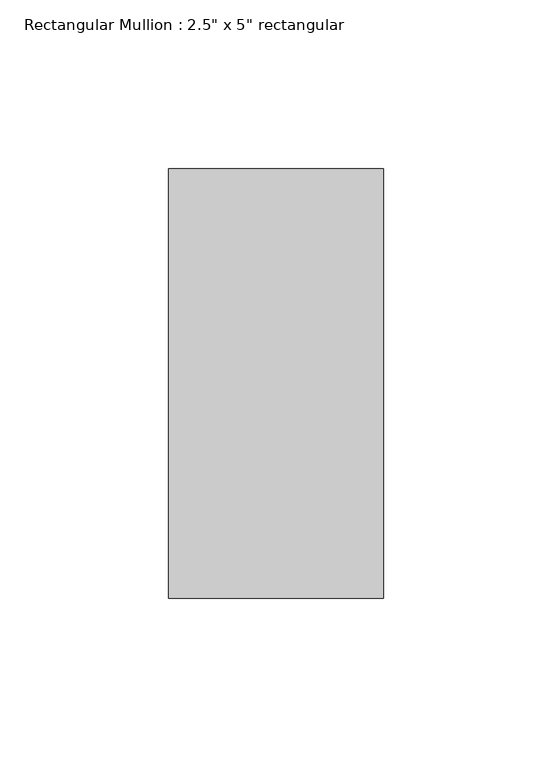
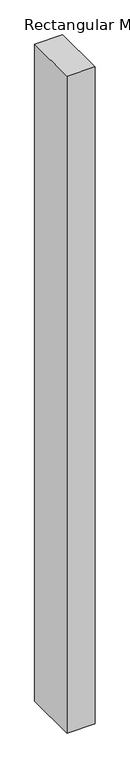
"""IFC4 building model written with IfcOpenShell, lengths in millimetres: member geometry."""

from ifc_helpers import new_model, si_unit, frame, origin, place, context, project, spatial, polyline, outline, extrude, source, transform, mapped, element, save


def member_f7325308(model_context):
    return source(origin(), model_context, "Body", "SweptSolid", [
        extrude(outline(polyline([(0.0, 63.5), (0.0, -63.5), (-63.5, -63.5), (-63.5, 63.5), (0.0, 63.5)])), frame((0.0, 0.0, -1578.2793787), z_axis=(0.0, 0.0, 1.0), x_axis=(1.0, 0.0, 0.0)), (0.0, 0.0, 1.0), 1578.2793787),
    ])


if __name__ == "__main__":
    model = new_model("IFC4")
    model_context = context("Model", 3, world=origin())
    ifc_project = project(units=[si_unit("LENGTHUNIT", "METRE", prefix="MILLI")], contexts=[model_context])
    site = spatial("IfcSite", under=ifc_project)
    building = spatial("IfcBuilding", under=site)
    placement = place(None, origin())
    member_shape = member_f7325308(model_context)
    element("IfcMember", 1, ObjectType="Rectangular Mullion : 2.5\" x 5\" rectangular", at=placement, inside=building, context=model_context, shape_type="MappedRepresentation", body=[
        mapped(member_shape, transform((0.0, 0.0, 0.0), x_axis=(1.0, 0.0, 0.0), y_axis=(0.0, 1.0, 0.0), z_axis=(0.0, 0.0, 1.0))),
    ])
    save(model, "model.ifc")

# Revit data of these elements
# Type "Rectangular Mullion : 2.5\" x 5\" rectangular"
#   built-in parameter 1007304 = 0.416667 (stored number, unit not read)
#   built-in parameter 1007301 = 0.104167 (stored number, unit not read)
#   built-in parameter 1007300 = 0.104167 (stored number, unit not read)
# Element 1 (IfcMember, "Rectangular Mullion : 2.5\" x 5\" rectangular")
#   Materials on its faces: "Aluminum"
# Materials
#   "Aluminum": class "Metal", colour RGB 247 247 247, transparency 0, Description = "Aluminum 6061", Cost = 0
